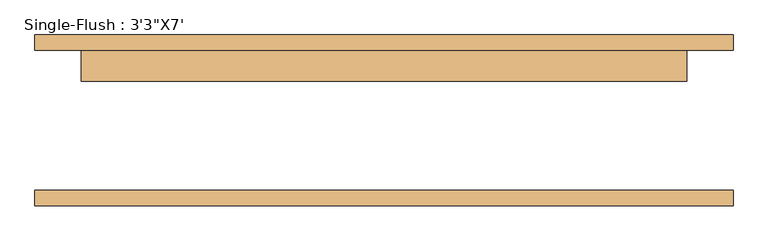
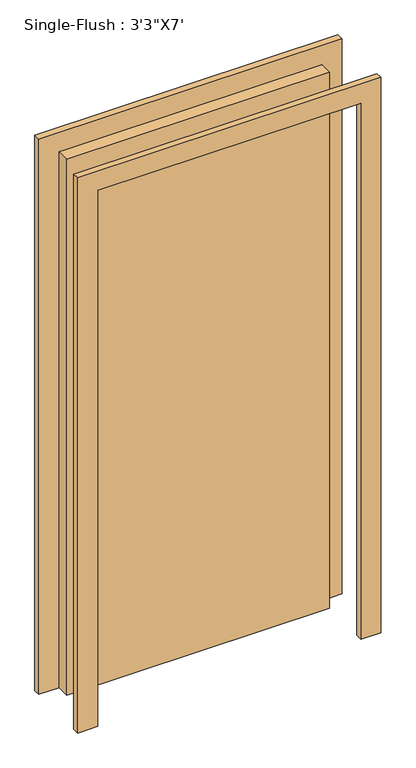
"""IFC4 building model written with IfcOpenShell, lengths in millimetres: door geometry."""

from ifc_helpers import new_model, si_unit, frame, origin, origin_with_axes, place, context, project, spatial, polyline, outline, extrude, source, transform, mapped, element, save


def door_ddcbdd8b(model_context):
    return source(origin(), model_context, "Body", "SweptSolid", [
        extrude(outline(polyline([(2209.8, -571.5), (0.0, -571.5), (0.0, -495.3), (2133.6, -495.3), (2133.6, 495.3), (0.0, 495.3), (0.0, 571.5), (2209.8, 571.5), (2209.8, -571.5)])), frame((0.0, 114.3, 0.0), z_axis=(0.0, 1.0, 0.0), x_axis=(0.0, 0.0, 1.0)), (0.0, 0.0, 1.0), 25.4),
        extrude(outline(polyline([(2209.8, 571.5), (2209.8, -571.5), (0.0, -571.5), (0.0, -495.3), (2133.6, -495.3), (2133.6, 495.3), (0.0, 495.3), (0.0, 571.5), (2209.8, 571.5)])), frame((0.0, -139.7, 0.0), z_axis=(0.0, 1.0, 0.0), x_axis=(0.0, 0.0, 1.0)), (0.0, 0.0, 1.0), 25.4),
        extrude(outline(polyline([(495.3, 63.5), (-495.3, 63.5), (-495.3, 114.3), (495.3, 114.3), (495.3, 63.5)])), origin_with_axes(), (0.0, 0.0, 1.0), 2133.6),
    ])


if __name__ == "__main__":
    model = new_model("IFC4")
    model_context = context("Model", 3, world=origin())
    ifc_project = project(units=[si_unit("LENGTHUNIT", "METRE", prefix="MILLI")], contexts=[model_context])
    site = spatial("IfcSite", under=ifc_project)
    building = spatial("IfcBuilding", under=site)
    placement = place(None, origin())
    door_shape = door_ddcbdd8b(model_context)
    element("IfcDoor", 1, ObjectType="Single-Flush : 3'3\"X7'", at=placement, inside=building, context=model_context, shape_type="MappedRepresentation", body=[
        mapped(door_shape, transform((0.0, 0.0, 0.0), x_axis=(1.0, 0.0, 0.0), y_axis=(0.0, 1.0, 0.0), z_axis=(0.0, 0.0, 1.0))),
    ])
    save(model, "model.ifc")

# Revit data of these elements
# Type "Single-Flush : 3'3\"X7'"
#   Type Mark = "11"
#   Construction Type Id = "MDOOR"
#   Assembly Code = "C1020"
#   Analytic Construction = "Metal"
#   Thickness = 0' - 2"
#   Heat Transfer Coefficient (U) = 0.651978 BTU/(h·ft²·°F)
#   Height = 7' - 0"
#   Trim Projection Ext = 0' - 1"
#   Trim Projection Int = 0' - 1"
#   Trim Width = 0' - 3"
#   Width = 3' - 3"
#   Define Thermal Properties by = 1
#   Door Material = Door - Panel
#   Frame Material = Door - Frame
#   Visual Light Transmittance = 0
#   Solar Heat Gain Coefficient = 0
#   Function = (empty or 0)
#   Wall Closure = (empty or 0)
# Element 1 (IfcDoor, "Single-Flush : 3'3\"X7'")
#   Materials on its faces: "Door - Frame", "Door - Panel"
# Materials
#   "Door - Panel": class "Wood", colour RGB 210 159 95, transparency 0, Cost = 0
#   "Door - Frame": colour RGB 118 70 51, transparency 0, Cost = 0
